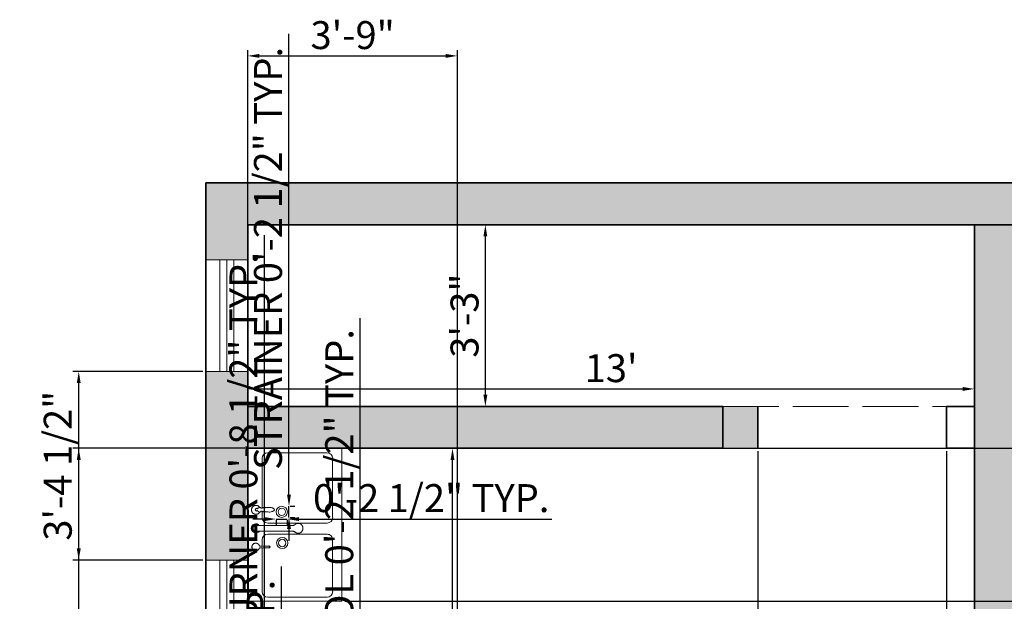
# Model space of a CAD drawing. Units: inches. Extents: x -40 to 424, y -33 to 568.
# Tile 6 of 8: x -40 to 171, y 438 to 563. Entities that reach past the tile are written whole.
import ezdxf

# ---------------------------------------------------------------- set-up
doc = ezdxf.new("R2010")
doc.units = ezdxf.units.IN
doc.linetypes.add('ACAD_ISO02W100', pattern=[15, 12, -3])
for name, color, linetype, lineweight in [('A-ANNO-DIMS', 7, 'Continuous', 18), ('A-FLOR-FIXT', 7, 'Continuous', 18), ('A-GLAZ', 7, 'Continuous', 18), ('A-WALL-OVHD', 7, 'ACAD_ISO02W100', 18), ('A-WALL-PATT', 30, 'Continuous', 13), ('wall', 7, 'Continuous', 35)]:
    doc.layers.add(name, color=color, linetype=linetype, lineweight=lineweight)
doc.styles.get("Standard").update_dxf_attribs({"font": 'arial.ttf'})
doc.dimstyles.new('ISO-25', dxfattribs={"dimtxt": 6, "dimasz": 2.5, "dimexe": 1.25, "dimexo": 0.625, "dimtad": 1, "dimdec": 1, "dimlunit": 3, "dimtxsty": 'Standard', "dimcen": 2.5, "dimadec": 0, "dimazin": 0, "dimtfac": 1, "dimtdec": 1, "dimtmove": 0, "dimatfit": 3, "dimfxl": 1, "dimarcsym": 0})

# ---------------------------------------------------------------- blocks, each defined once
blk = doc.blocks.new('*D27')
at = {"layer": 'A-ANNO-DIMS', "color": 0, "lineweight": -2, "transparency": 16777216}
for p, q in [((52.32, 471), (51.7, 471)), ((52.95, 281.5), (52.95, 468.5)), ((53.57, 279), (54.2, 279))]:
    blk.add_line(p, q, dxfattribs=at)
at = {"layer": 'A-ANNO-DIMS', "color": 0, "transparency": 16777216}
for points in [[(52.53, 468.5), (53.36, 468.5), (52.95, 471)], [(52.53, 281.5), (53.36, 281.5), (52.95, 279)]]:
    blk.add_solid(points, dxfattribs=at)
at = {"layer": 'Defpoints', "color": 0, "transparency": 16777216}
for p in [(52.95, 471), (52.95, 471), (52.95, 279)]:
    blk.add_point(p, dxfattribs=at)
at = {"layer": 'A-ANNO-DIMS', "color": 0, "transparency": 16777216, "insert": (49.26, 375), "char_height": 6, "attachment_point": 5, "rotation": 90}
blk.add_mtext("16'", dxfattribs=at)
blk = doc.blocks.new('*D28')
at = {"layer": 'A-ANNO-DIMS', "color": 0, "lineweight": -2, "transparency": 16777216}
for p, q in [((9.08, 457.74), (9.08, 411.34)), ((165, 457.74), (165, 411.34)), ((11.58, 412.59), (162.5, 412.59))]:
    blk.add_line(p, q, dxfattribs=at)
at = {"layer": 'A-ANNO-DIMS', "color": 0, "transparency": 16777216}
for points in [[(11.58, 413.01), (11.58, 412.18), (9.08, 412.59)], [(162.5, 413.01), (162.5, 412.18), (165, 412.59)]]:
    blk.add_solid(points, dxfattribs=at)
at = {"layer": 'Defpoints', "color": 0, "transparency": 16777216}
for p in [(9.08, 458.36), (165, 458.36), (165, 412.59)]:
    blk.add_point(p, dxfattribs=at)
at = {"layer": 'A-ANNO-DIMS', "color": 0, "transparency": 16777216, "insert": (87.04, 416.28), "char_height": 6, "attachment_point": 5}
blk.add_mtext('12\'-11.9"', dxfattribs=at)
blk = doc.blocks.new('*D29')
at = {"layer": 'A-ANNO-DIMS', "color": 0, "lineweight": -2, "transparency": 16777216}
for p, q in [((59.38, 519), (58.75, 519)), ((60, 482.5), (60, 516.5)), ((59.38, 480), (58.75, 480))]:
    blk.add_line(p, q, dxfattribs=at)
at = {"layer": 'A-ANNO-DIMS', "color": 0, "transparency": 16777216}
for points in [[(59.58, 516.5), (60.42, 516.5), (60, 519)], [(59.58, 482.5), (60.42, 482.5), (60, 480)]]:
    blk.add_solid(points, dxfattribs=at)
at = {"layer": 'Defpoints', "color": 0, "transparency": 16777216}
for p in [(60, 519), (60, 519), (60, 480)]:
    blk.add_point(p, dxfattribs=at)
at = {"layer": 'A-ANNO-DIMS', "color": 0, "transparency": 16777216, "insert": (56.31, 499.5), "char_height": 6, "attachment_point": 5, "rotation": 90}
blk.add_mtext('3\'-3"', dxfattribs=at)
blk = doc.blocks.new('*D30')
at = {"layer": 'A-ANNO-DIMS', "color": 0, "lineweight": -2, "transparency": 16777216}
for p, q in [((9, 510.87), (9, 482.5)), ((165, 510.87), (165, 482.5)), ((11.5, 483.75), (162.5, 483.75))]:
    blk.add_line(p, q, dxfattribs=at)
at = {"layer": 'A-ANNO-DIMS', "color": 0, "transparency": 16777216}
for points in [[(11.5, 484.17), (11.5, 483.33), (9, 483.75)], [(162.5, 484.17), (162.5, 483.33), (165, 483.75)]]:
    blk.add_solid(points, dxfattribs=at)
at = {"layer": 'Defpoints', "color": 0, "transparency": 16777216}
for p in [(9, 511.5), (165, 511.5), (165, 483.75)]:
    blk.add_point(p, dxfattribs=at)
at = {"layer": 'A-ANNO-DIMS', "color": 0, "transparency": 16777216, "insert": (87, 487.44), "char_height": 6, "attachment_point": 5}
blk.add_mtext("13'", dxfattribs=at)
blk = doc.blocks.new('WIN-48IN')
for p, q in [((0, 0), (0, 9)), ((48, 0), (48, 9)), ((0, 6), (48, 6)), ((0, 4.5), (48, 4.5)), ((0, 3), (48, 3))]:
    blk.add_line(p, q)
blk = doc.blocks.new('WIN-24IN')
for p, q in [((9, 24), (0, 24)), ((3, 0), (3, 24)), ((4.5, 0), (4.5, 24)), ((6, 0), (6, 24)), ((9, 0), (0, 0))]:
    blk.add_line(p, q)
blk = doc.blocks.new('SINK-STRAINER')
for radius in [1.2, 0.798]:
    blk.add_circle((1.2, 1.2), radius)
blk = doc.blocks.new('*D43')
at = {"layer": 'A-ANNO-DIMS', "color": 0, "lineweight": -2, "transparency": 16777216}
for p, q in [((16.2, 351), (16.2, 445.58)), ((9.62, 351), (17.45, 351)), ((16.2, 305.5), (16.2, 348.5)), ((9.62, 303), (17.45, 303))]:
    blk.add_line(p, q, dxfattribs=at)
at = {"layer": 'A-ANNO-DIMS', "color": 0, "transparency": 16777216}
for points in [[(15.78, 348.5), (16.62, 348.5), (16.2, 351)], [(15.78, 305.5), (16.62, 305.5), (16.2, 303)]]:
    blk.add_solid(points, dxfattribs=at)
at = {"layer": 'Defpoints', "color": 0, "transparency": 16777216}
for p in [(9, 351), (16.2, 351), (9, 303)]:
    blk.add_point(p, dxfattribs=at)
at = {"layer": 'A-ANNO-DIMS', "color": 0, "transparency": 16777216, "insert": (12.47, 399.54), "char_height": 6, "attachment_point": 5, "rotation": 90}
blk.add_mtext('WINDOW W1 4\'-0" TYP.', dxfattribs=at)
blk = doc.blocks.new('*D71')
at = {"layer": 'A-ANNO-DIMS', "color": 0, "lineweight": -2, "transparency": 16777216}
for p, q in [((33.12, 401.38), (33.12, 498.92)), ((32.88, 398.88), (31.88, 398.88)), ((33.12, 396.38), (33.12, 398.88)), ((32.88, 396.38), (31.88, 396.38)), ((33.12, 393.88), (33.12, 391.38))]:
    blk.add_line(p, q, dxfattribs=at)
at = {"layer": 'A-ANNO-DIMS', "color": 0, "transparency": 16777216}
for points in [[(32.71, 401.38), (33.54, 401.38), (33.12, 398.88)], [(32.71, 393.88), (33.54, 393.88), (33.12, 396.38)]]:
    blk.add_solid(points, dxfattribs=at)
at = {"layer": 'Defpoints', "color": 0, "transparency": 16777216}
for p in [(33.12, 398.88), (33.5, 398.88), (33.5, 396.38)]:
    blk.add_point(p, dxfattribs=at)
at = {"layer": 'A-ANNO-DIMS', "color": 0, "transparency": 16777216, "insert": (29.4, 451.4), "char_height": 6, "attachment_point": 5, "rotation": 90}
blk.add_mtext('CONTROL 0\'-2 1/2" TYP.', dxfattribs=at)
blk = doc.blocks.new('*D75')
at = {"layer": 'A-ANNO-DIMS', "color": 0, "lineweight": -2, "transparency": 16777216}
for p, q in [((12.57, 399.46), (12.57, 516.79)), ((13.25, 399.46), (11.32, 399.46)), ((12.57, 393.29), (12.57, 396.96)), ((13.25, 390.79), (11.32, 390.79))]:
    blk.add_line(p, q, dxfattribs=at)
at = {"layer": 'A-ANNO-DIMS', "color": 0, "transparency": 16777216}
for points in [[(12.15, 396.96), (12.99, 396.96), (12.57, 399.46)], [(12.15, 393.29), (12.99, 393.29), (12.57, 390.79)]]:
    blk.add_solid(points, dxfattribs=at)
at = {"layer": 'Defpoints', "color": 0, "transparency": 16777216}
for p in [(12.57, 399.46), (13.87, 399.46), (13.87, 390.79)]:
    blk.add_point(p, dxfattribs=at)
at = {"layer": 'A-ANNO-DIMS', "color": 0, "transparency": 16777216, "insert": (8.84, 459.38), "char_height": 6, "attachment_point": 5, "rotation": 90}
blk.add_mtext('REAR BURNER 0\'-8 1/2" TYP.', dxfattribs=at)
blk = doc.blocks.new('*D77')
at = {"layer": 'A-ANNO-DIMS', "color": 0, "lineweight": -2, "transparency": 16777216}
for p, q in [((17.84, 461.05), (17.84, 560.03)), ((17.84, 456.15), (17.84, 458.55)), ((18.11, 458.55), (19.09, 458.55)), ((18.11, 456.15), (19.09, 456.15)), ((17.84, 453.65), (17.84, 451.15))]:
    blk.add_line(p, q, dxfattribs=at)
at = {"layer": 'A-ANNO-DIMS', "color": 0, "transparency": 16777216}
for points in [[(17.42, 461.05), (18.26, 461.05), (17.84, 458.55)], [(17.42, 453.65), (18.26, 453.65), (17.84, 456.15)]]:
    blk.add_solid(points, dxfattribs=at)
at = {"layer": 'Defpoints', "color": 0, "transparency": 16777216}
for p in [(17.48, 458.55), (17.84, 458.55), (17.48, 456.15)]:
    blk.add_point(p, dxfattribs=at)
at = {"layer": 'A-ANNO-DIMS', "color": 0, "transparency": 16777216, "insert": (14.11, 511.79), "char_height": 6, "attachment_point": 5, "rotation": 90}
blk.add_mtext('STRAINER 0\'-2 1/2" TYP.', dxfattribs=at)
blk = doc.blocks.new('*D78')
at = {"layer": 'A-ANNO-DIMS', "color": 0, "lineweight": -2, "transparency": 16777216}
for p, q in [((12.59, 455.8), (10.09, 455.8)), ((15.09, 455.8), (17.48, 455.8)), ((15.09, 455.53), (15.09, 454.55)), ((17.48, 455.53), (17.48, 454.55)), ((19.98, 455.8), (74.29, 455.8))]:
    blk.add_line(p, q, dxfattribs=at)
at = {"layer": 'A-ANNO-DIMS', "color": 0, "transparency": 16777216}
for points in [[(12.59, 456.21), (12.59, 455.38), (15.09, 455.8)], [(19.98, 456.21), (19.98, 455.38), (17.48, 455.8)]]:
    blk.add_solid(points, dxfattribs=at)
at = {"layer": 'Defpoints', "color": 0, "transparency": 16777216}
for p in [(15.09, 456.15), (17.48, 456.15), (17.48, 455.8)]:
    blk.add_point(p, dxfattribs=at)
at = {"layer": 'A-ANNO-DIMS', "color": 0, "transparency": 16777216, "insert": (48.38, 459.52), "char_height": 6, "attachment_point": 5}
blk.add_mtext('0\'-2 1/2" TYP.', dxfattribs=at)
blk = doc.blocks.new('*D85')
at = {"layer": 'A-ANNO-DIMS', "color": 0, "lineweight": -2, "transparency": 16777216}
for p, q in [((-0.63, 487.5), (-28.55, 487.5)), ((-27.3, 449.5), (-27.3, 485)), ((-0.63, 447), (-28.55, 447))]:
    blk.add_line(p, q, dxfattribs=at)
at = {"layer": 'A-ANNO-DIMS', "color": 0, "transparency": 16777216}
for points in [[(-27.72, 485), (-26.88, 485), (-27.3, 487.5)], [(-27.72, 449.5), (-26.88, 449.5), (-27.3, 447)]]:
    blk.add_solid(points, dxfattribs=at)
at = {"layer": 'Defpoints', "color": 0, "transparency": 16777216}
for p in [(-27.3, 487.5), (0, 487.5), (0, 447)]:
    blk.add_point(p, dxfattribs=at)
at = {"layer": 'A-ANNO-DIMS', "color": 0, "transparency": 16777216, "insert": (-31.03, 467.25), "char_height": 6, "attachment_point": 5, "rotation": 90}
blk.add_mtext('3\'-4 1/2"', dxfattribs=at)
blk = doc.blocks.new('*D91')
at = {"layer": 'A-ANNO-DIMS', "color": 0, "lineweight": -2, "transparency": 16777216}
for p, q in [((9, 90.62), (9, 556.55)), ((54, 90.62), (54, 556.55)), ((11.5, 555.3), (51.5, 555.3))]:
    blk.add_line(p, q, dxfattribs=at)
at = {"layer": 'A-ANNO-DIMS', "color": 0, "transparency": 16777216}
for points in [[(11.5, 555.72), (11.5, 554.88), (9, 555.3)], [(51.5, 555.72), (51.5, 554.88), (54, 555.3)]]:
    blk.add_solid(points, dxfattribs=at)
at = {"layer": 'Defpoints', "color": 0, "transparency": 16777216}
for p in [(54, 555.3), (9, 90), (54, 90)]:
    blk.add_point(p, dxfattribs=at)
at = {"layer": 'A-ANNO-DIMS', "color": 0, "transparency": 16777216, "insert": (31.5, 558.99), "char_height": 6, "attachment_point": 5}
blk.add_mtext('3\'-9"', dxfattribs=at)
blk = doc.blocks.new('*D92')
at = {"layer": 'A-ANNO-DIMS', "color": 0, "lineweight": -2, "transparency": 16777216}
for p, q in [((118.47, 470.38), (118.47, -28.55)), ((159, 470.38), (159, -28.55)), ((120.97, -27.3), (156.5, -27.3))]:
    blk.add_line(p, q, dxfattribs=at)
at = {"layer": 'A-ANNO-DIMS', "color": 0, "transparency": 16777216}
for points in [[(120.97, -26.88), (120.97, -27.72), (118.47, -27.3)], [(156.5, -26.88), (156.5, -27.72), (159, -27.3)]]:
    blk.add_solid(points, dxfattribs=at)
at = {"layer": 'Defpoints', "color": 0, "transparency": 16777216}
for p in [(118.47, 471), (159, 471), (159, -27.3)]:
    blk.add_point(p, dxfattribs=at)
at = {"layer": 'A-ANNO-DIMS', "color": 0, "transparency": 16777216, "insert": (138.73, -23.57), "char_height": 6, "attachment_point": 5}
blk.add_mtext('3\'-4 1/2"', dxfattribs=at)
blk = doc.blocks.new('*D100')
at = {"layer": 'A-ANNO-DIMS', "color": 0, "lineweight": -2, "transparency": 16777216}
for p, q in [((8.37, 471), (-28.55, 471)), ((-27.3, 360.94), (-27.3, 468.5)), ((8.37, 358.44), (-28.55, 358.44))]:
    blk.add_line(p, q, dxfattribs=at)
at = {"layer": 'A-ANNO-DIMS', "color": 0, "transparency": 16777216}
for points in [[(-27.72, 468.5), (-26.88, 468.5), (-27.3, 471)], [(-27.72, 360.94), (-26.88, 360.94), (-27.3, 358.44)]]:
    blk.add_solid(points, dxfattribs=at)
at = {"layer": 'Defpoints', "color": 0, "transparency": 16777216}
for p in [(-27.3, 471), (9, 471), (9, 358.44)]:
    blk.add_point(p, dxfattribs=at)
at = {"layer": 'A-ANNO-DIMS', "color": 0, "transparency": 16777216, "insert": (-31.03, 414.72), "char_height": 6, "attachment_point": 5, "rotation": 90}
blk.add_mtext('9\'-4 1/2"', dxfattribs=at)
blk = doc.blocks.new('*D102')
at = {"layer": 'A-ANNO-DIMS', "color": 0, "lineweight": -2, "transparency": 16777216}
for p, q in [((29.83, 471), (412.55, 471)), ((411.3, 440.63), (411.3, 468.5)), ((29.83, 438.13), (412.55, 438.13))]:
    blk.add_line(p, q, dxfattribs=at)
at = {"layer": 'A-ANNO-DIMS', "color": 0, "transparency": 16777216}
for points in [[(410.88, 468.5), (411.72, 468.5), (411.3, 471)], [(410.88, 440.63), (411.72, 440.63), (411.3, 438.13)]]:
    blk.add_solid(points, dxfattribs=at)
at = {"layer": 'Defpoints', "color": 0, "transparency": 16777216}
for p in [(29.21, 471), (411.3, 471), (29.21, 438.13)]:
    blk.add_point(p, dxfattribs=at)
at = {"layer": 'A-ANNO-DIMS', "color": 0, "transparency": 16777216, "insert": (407.61, 454.56), "char_height": 6, "attachment_point": 5, "rotation": 90}
blk.add_mtext('2\'-9"', dxfattribs=at)

msp = doc.modelspace()

# ---------------------------------------------------------------- hatches: boundary and pattern name
at = {"layer": 'A-WALL-PATT'}
h = msp.add_hatch(color=256, dxfattribs=at)
h.dxf.hatch_style = 1
h.paths.add_polyline_path([(9, 399), (0, 399), (0, 351), (9, 351)])
h.paths.add_polyline_path([(9, 303), (0, 303), (0, 210), (9, 210)])
h.paths.add_polyline_path([(9, 150), (0, 150), (0, 0), (384, 0), (384, 69), (375, 69), (375, 62.24), (375, 9), (9, 9)])
h.paths.add_polyline_path([(210, 177), (216, 177), (216, 186), (210, 186), (210, 216), (201, 216), (201, 90), (195, 90), (195, 81), (201, 81), (201, 9), (210, 9)])
h.paths.add_polyline_path([(384, 216), (375, 216), (375, 117), (384, 117)])
h.paths.add_polyline_path([(384, 298.5), (375, 298.5), (375, 279), (375, 240), (384, 240)])
h.paths.add_polyline_path([(384, 417), (375, 417), (375, 334.5), (384, 334.5)])
h.paths.add_polyline_path([(384, 528), (216, 528), (216, 519), (375, 519), (375, 465), (384, 465)])
h.paths.add_polyline_path([(192, 528), (0, 528), (0, 511.5), (9, 511.5), (9, 519), (192, 519)])
h.paths.add_polyline_path([(9, 487.5), (0, 487.5), (0, 447), (9, 447)])
h.paths.add_polyline_path([(111, 480), (9, 480), (9, 471), (111, 471)])
h.paths.add_polyline_path([(174, 519), (165, 519), (165, 354), (174, 354)])
h.paths.add_polyline_path([(243, 426), (237.86, 426), (234, 426), (234, 420), (174, 420), (174, 411), (234, 411), (234, 405), (239.14, 405), (243, 405)])
h.paths.add_polyline_path([(243, 519), (234, 519), (234, 460.14, -0.031638), (237.86, 460.2), (237.86, 462), (243, 462)])
h.paths.add_polyline_path([(243, 369), (234, 369), (234, 354), (375, 354), (375, 363), (243, 363)])
h.paths.add_polyline_path([(375, 279), (195, 279), (195, 270), (201, 270), (201, 264), (210, 264), (210, 270), (375, 270)])
h.paths.add_polyline_path([(291, 270), (282, 270), (282, 222), (286.29, 222), (291, 222)])
h.paths.add_polyline_path([(375, 186), (291, 186), (291, 192), (282, 192), (282, 186), (252, 186), (252, 180.86), (252, 177), (375, 177)])
h.paths.add_polyline_path([(147, 279), (9, 279), (9, 270), (147, 270)])
h = msp.add_hatch(color=256, dxfattribs=at)
h.dxf.hatch_style = 1
h.paths.add_polyline_path([(118.47, 480), (111, 480), (111, 471), (118.47, 471)])

# ---------------------------------------------------------------- linework, layer by layer
at = {"layer": 'A-FLOR-FIXT'}
for p, q in [((13.29, 470.05), (22.39, 470.05)), ((22.39, 470.05), (26.02, 470.05)), ((12.09, 458.15), (12.09, 468.85)), ((27.21, 468.85), (27.21, 456.13)), ((10.64, 457.91), (10.58, 457.81)), ((10.58, 457.81), (10.58, 457.81)), ((10.64, 457.71), (10.58, 457.81)), ((10.58, 457.81), (10.58, 457.81)), ((10.58, 457.81), (10.58, 457.81)), ((10.66, 457.93), (10.64, 457.91)), ((10.66, 457.69), (10.64, 457.71)), ((10.82, 458.05), (10.66, 457.93)), ((10.82, 457.57), (10.66, 457.69)), ((10.83, 458.05), (10.82, 458.05)), ((10.83, 457.56), (10.82, 457.57)), ((10.88, 458.09), (10.83, 458.05)), ((10.88, 457.53), (10.83, 457.56)), ((10.93, 458.11), (10.88, 458.09)), ((10.93, 457.51), (10.88, 457.53)), ((11, 458.05), (10.93, 458.11)), ((11, 457.56), (10.93, 457.51)), ((11.01, 458.05), (11, 458.05)), ((11.01, 457.57), (11, 457.56)), ((11.06, 458.01), (11.01, 458.05)), ((11.06, 457.61), (11.01, 457.57)), ((11.07, 458.01), (11.06, 458.01)), ((11.07, 457.61), (11.06, 457.61)), ((11.11, 458.01), (11.07, 458.01)), ((11.11, 457.61), (11.07, 457.61)), ((11.17, 458.1), (11.11, 458.01)), ((11.17, 457.52), (11.11, 457.61)), ((11.21, 458.16), (11.17, 458.1)), ((11.21, 457.46), (11.17, 457.52)), ((11.24, 458.2), (11.21, 458.16)), ((11.24, 457.42), (11.21, 457.46)), ((11.26, 458.22), (11.24, 458.21)), ((11.24, 458.21), (11.24, 458.2)), ((11.24, 457.41), (11.24, 457.42)), ((11.26, 457.4), (11.24, 457.41)), ((11.27, 458.22), (11.26, 458.22)), ((11.27, 457.4), (11.26, 457.4)), ((11.41, 458.28), (11.27, 458.22)), ((11.41, 457.34), (11.27, 457.4)), ((11.46, 458.31), (11.41, 458.28)), ((11.42, 457.33), (11.41, 457.34)), ((11.43, 457.33), (11.42, 457.33)), ((11.42, 457.33), (11.42, 457.33)), ((11.46, 457.31), (11.43, 457.33)), ((11.46, 458.31), (11.46, 458.31)), ((11.65, 458.28), (11.46, 458.31)), ((11.65, 457.34), (11.46, 457.31)), ((11.46, 457.31), (11.46, 457.31)), ((11.46, 457.31), (11.46, 457.31)), ((11.66, 458.28), (11.65, 458.28)), ((11.66, 457.34), (11.65, 457.34)), ((11.68, 458.28), (11.66, 458.28)), ((11.68, 457.34), (11.66, 457.34)), ((11.7, 458.28), (11.68, 458.28)), ((11.7, 457.34), (11.68, 457.34)), ((11.86, 458.15), (11.7, 458.28)), ((11.89, 457.49), (11.7, 457.34)), ((11.89, 458.13), (11.86, 458.15)), ((11.99, 458.12), (11.89, 458.13)), ((11.95, 457.49), (11.89, 457.49)), ((11.99, 457.49), (11.95, 457.49)), ((12.1, 458.16), (11.99, 458.12)), ((12.08, 457.47), (11.99, 457.49)), ((12.1, 457.46), (12.08, 457.47)), ((12.09, 456.13), (12.09, 457.46)), ((12.18, 458.18), (12.1, 458.16)), ((12.18, 457.44), (12.1, 457.46)), ((12.26, 458.27), (12.18, 458.18)), ((12.26, 457.35), (12.18, 457.44)), ((12.29, 458.27), (12.26, 458.27)), ((12.29, 457.35), (12.26, 457.35)), ((12.4, 458.19), (12.29, 458.27)), ((12.4, 457.43), (12.29, 457.35)), ((12.29, 457.35), (12.29, 457.35)), ((12.46, 458.2), (12.4, 458.19)), ((12.63, 457.39), (12.4, 457.43)), ((12.58, 458.22), (12.46, 458.2)), ((12.6, 458.22), (12.58, 458.22)), ((12.64, 458.23), (12.6, 458.22)), ((12.71, 457.38), (12.63, 457.39)), ((12.66, 458.23), (12.64, 458.23)), ((12.71, 458.24), (12.66, 458.23)), ((12.72, 458.24), (12.71, 458.24)), ((12.75, 457.37), (12.71, 457.38)), ((12.76, 458.25), (12.72, 458.24)), ((12.79, 457.36), (12.75, 457.37)), ((12.81, 458.26), (12.76, 458.25)), ((12.87, 457.35), (12.79, 457.36)), ((12.9, 458.27), (12.81, 458.26)), ((12.88, 457.35), (12.87, 457.35)), ((12.9, 457.35), (12.88, 457.35)), ((12.94, 458.28), (12.9, 458.27)), ((12.93, 457.34), (12.9, 457.35)), ((12.94, 457.34), (12.93, 457.34)), ((13.36, 458.3), (12.94, 458.28)), ((13.04, 457.34), (12.94, 457.34)), ((13.05, 457.34), (13.04, 457.34)), ((13.08, 457.33), (13.05, 457.34)), ((13.26, 457.32), (13.08, 457.33)), ((13.36, 457.32), (13.26, 457.32)), ((13.37, 458.3), (13.36, 458.3)), ((13.58, 457.31), (13.36, 457.32)), ((13.51, 458.3), (13.37, 458.3)), ((13.52, 458.3), (13.51, 458.3)), ((13.55, 458.31), (13.52, 458.3)), ((13.7, 458.31), (13.55, 458.31)), ((13.7, 457.31), (13.58, 457.31)), ((13.7, 458.31), (13.7, 458.31)), ((13.78, 458.3), (13.7, 458.31)), ((14.02, 457.36), (13.7, 457.31)), ((13.79, 458.29), (13.78, 458.3)), ((13.83, 458.29), (13.79, 458.29)), ((13.79, 458.29), (13.79, 458.29)), ((13.85, 458.28), (13.83, 458.29)), ((14.02, 458.26), (13.85, 458.28)), ((14.13, 458.23), (14.02, 458.26)), ((14.16, 457.4), (14.02, 457.36)), ((14.22, 458.2), (14.13, 458.23)), ((14.27, 457.43), (14.16, 457.4)), ((14.27, 458.19), (14.22, 458.2)), ((14.37, 458.14), (14.27, 458.19)), ((14.51, 457.53), (14.27, 457.43)), ((14.46, 458.11), (14.37, 458.14)), ((14.51, 458.09), (14.46, 458.11)), ((14.6, 458.01), (14.51, 458.09)), ((14.58, 457.59), (14.51, 457.53)), ((14.68, 457.67), (14.58, 457.59)), ((14.65, 457.98), (14.6, 458.01)), ((14.68, 457.95), (14.65, 457.98)), ((14.69, 457.89), (14.68, 457.95)), ((14.69, 457.7), (14.68, 457.67)), ((14.71, 457.81), (14.69, 457.89)), ((14.7, 457.77), (14.69, 457.7)), ((14.71, 457.81), (14.7, 457.77)), ((22.39, 454.93), (13.29, 454.93)), ((26.02, 454.93), (22.39, 454.93)), ((10.7, 454.4), (10.83, 454.4)), ((10.73, 453.22), (10.81, 453.22)), ((10.81, 453.22), (10.83, 453.22)), ((10.83, 454.4), (10.86, 454.4)), ((10.83, 453.22), (10.86, 453.22)), ((10.86, 454.4), (10.94, 454.4)), ((10.86, 453.22), (10.94, 453.22)), ((10.94, 454.4), (11, 454.4)), ((10.94, 453.22), (10.95, 453.22)), ((10.95, 453.22), (10.96, 453.22)), ((10.96, 453.22), (11, 453.22)), ((11, 454.4), (11.02, 454.4)), ((11, 453.22), (11.02, 453.22)), ((11.02, 454.4), (11.15, 454.4)), ((11.02, 453.22), (11.15, 453.22)), ((11.15, 454.4), (11.29, 454.4)), ((11.15, 453.22), (11.29, 453.22)), ((11.29, 454.4), (11.31, 454.4)), ((11.29, 453.22), (11.3, 453.22)), ((11.3, 453.22), (11.31, 453.22)), ((11.32, 454.41), (11.31, 454.4)), ((11.31, 454.4), (11.31, 454.4)), ((11.31, 453.22), (11.32, 453.22)), ((11.32, 454.41), (11.36, 454.4)), ((11.32, 453.22), (11.36, 453.22)), ((11.35, 454.41), (11.36, 454.4)), ((11.36, 454.4), (11.36, 454.4)), ((11.36, 454.4), (11.38, 454.4)), ((11.36, 453.22), (11.38, 453.22)), ((11.38, 454.4), (11.42, 454.4)), ((11.38, 453.22), (11.42, 453.22)), ((11.42, 454.4), (11.46, 454.4)), ((11.42, 453.22), (11.46, 453.22)), ((11.46, 454.4), (11.48, 454.4)), ((11.46, 453.22), (11.48, 453.22)), ((11.48, 454.4), (11.49, 454.4)), ((11.48, 453.22), (11.49, 453.22)), ((11.49, 454.42), (11.49, 454.4)), ((11.49, 454.4), (12.15, 454.4)), ((11.49, 454.4), (11.49, 454.4)), ((11.49, 454.4), (11.49, 454.4)), ((11.49, 453.22), (11.49, 453.22)), ((11.49, 453.22), (11.49, 453.22)), ((11.49, 453.22), (11.71, 453.22)), ((11.71, 453.22), (14.77, 453.22)), ((12.15, 454.4), (12.39, 454.4)), ((12.39, 454.4), (13.02, 454.4)), ((13.02, 454.4), (13.03, 454.4)), ((13.03, 454.4), (13.11, 454.4)), ((13.11, 454.4), (13.13, 454.4)), ((13.13, 454.4), (13.14, 454.4)), ((13.14, 454.4), (13.16, 454.4)), ((13.16, 454.4), (13.16, 454.4)), ((13.16, 454.4), (13.17, 454.4)), ((13.17, 454.4), (13.25, 454.4)), ((13.25, 454.4), (13.26, 454.4)), ((13.26, 454.4), (13.3, 454.4)), ((22.39, 452.54), (13.29, 452.54)), ((13.3, 454.4), (13.31, 454.4)), ((13.31, 454.4), (13.33, 454.4)), ((13.33, 454.4), (13.47, 454.4)), ((13.47, 454.4), (13.48, 454.4)), ((13.48, 454.4), (13.61, 454.4)), ((13.61, 454.4), (13.61, 454.4)), ((13.61, 454.4), (13.69, 454.4)), ((13.69, 454.4), (13.78, 454.4)), ((13.78, 454.4), (14.05, 454.4)), ((14.05, 454.4), (14.06, 454.4)), ((14.06, 454.4), (14.1, 454.4)), ((14.1, 454.4), (14.12, 454.4)), ((14.12, 454.4), (14.13, 454.4)), ((14.13, 454.4), (14.2, 454.4)), ((14.2, 454.4), (14.26, 454.4)), ((14.26, 454.4), (14.28, 454.4)), ((14.28, 454.4), (14.32, 454.4)), ((14.32, 454.4), (14.46, 454.4)), ((14.46, 454.4), (14.6, 454.4)), ((14.6, 454.4), (14.76, 454.4)), ((14.76, 454.4), (14.91, 454.4)), ((14.77, 453.22), (14.84, 453.22)), ((14.84, 453.22), (15.04, 453.22)), ((14.91, 454.4), (15.06, 454.4)), ((15.04, 453.22), (15.11, 453.22)), ((15.06, 454.4), (15.32, 454.4)), ((15.11, 453.22), (15.19, 453.22)), ((15.19, 453.22), (15.26, 453.22)), ((15.26, 453.22), (15.5, 453.22)), ((15.32, 454.4), (15.52, 454.4)), ((15.5, 453.22), (15.52, 453.22)), ((15.52, 454.4), (15.55, 454.4)), ((15.52, 453.22), (15.69, 453.22)), ((15.55, 454.4), (15.77, 454.4)), ((15.69, 453.22), (16.35, 453.22)), ((15.77, 454.4), (16.06, 454.4)), ((16.06, 454.4), (16.11, 454.4)), ((16.11, 454.4), (16.69, 454.4)), ((16.35, 453.22), (16.69, 453.22)), ((16.69, 454.4), (17.68, 454.4)), ((16.69, 453.22), (16.86, 453.22)), ((16.86, 453.22), (17.2, 453.22)), ((17.2, 453.22), (17.71, 453.22)), ((17.68, 454.4), (17.69, 454.4)), ((17.69, 454.4), (17.71, 454.4)), ((17.71, 454.4), (18.52, 454.4)), ((17.71, 453.22), (18.32, 453.22)), ((22.39, 452.54), (26.02, 452.54)), ((26.02, 452.54), (22.39, 452.54)), ((12.09, 451.34), (12.09, 449.98)), ((27.21, 440.21), (27.21, 451.34)), ((27.21, 451.34), (27.21, 449.69)), ((11.7, 449.98), (11.64, 449.98)), ((11.7, 449.64), (11.64, 449.64)), ((11.71, 449.98), (11.7, 449.98)), ((11.71, 449.64), (11.7, 449.64)), ((11.77, 449.98), (11.71, 449.98)), ((11.77, 449.64), (11.71, 449.64)), ((11.82, 449.98), (11.77, 449.98)), ((11.99, 449.64), (11.77, 449.64)), ((11.9, 449.98), (11.82, 449.98)), ((12.03, 449.98), (11.9, 449.98)), ((12.03, 449.64), (11.99, 449.64)), ((12.31, 449.98), (12.03, 449.98)), ((12.05, 449.64), (12.03, 449.64)), ((12.35, 449.64), (12.05, 449.64)), ((12.09, 449.64), (12.09, 440.21)), ((12.35, 449.98), (12.31, 449.98)), ((12.64, 449.98), (12.35, 449.98)), ((12.62, 449.64), (12.35, 449.64)), ((12.64, 449.64), (12.62, 449.64)), ((12.69, 449.98), (12.64, 449.98)), ((12.67, 449.64), (12.64, 449.64)), ((12.72, 449.64), (12.67, 449.64)), ((12.72, 449.98), (12.69, 449.98)), ((12.78, 449.98), (12.72, 449.98)), ((12.82, 449.64), (12.72, 449.64)), ((12.85, 449.98), (12.78, 449.98)), ((12.9, 449.64), (12.82, 449.64)), ((12.82, 449.64), (12.82, 449.64)), ((12.82, 449.64), (12.82, 449.64)), ((12.87, 449.98), (12.85, 449.98)), ((12.96, 449.98), (12.87, 449.98)), ((12.95, 449.64), (12.9, 449.64)), ((12.97, 449.64), (12.95, 449.64)), ((12.97, 449.98), (12.96, 449.98)), ((12.98, 449.98), (12.97, 449.98)), ((13.04, 449.64), (12.97, 449.64)), ((13.1, 449.98), (12.98, 449.98)), ((13.18, 449.64), (13.04, 449.64)), ((13.27, 449.98), (13.1, 449.98)), ((13.2, 449.64), (13.18, 449.64)), ((13.24, 449.64), (13.2, 449.64)), ((13.27, 449.64), (13.24, 449.64)), ((13.27, 449.98), (13.27, 449.98)), ((13.33, 449.98), (13.27, 449.98)), ((13.28, 449.64), (13.27, 449.64)), ((13.47, 449.64), (13.28, 449.64)), ((13.35, 449.98), (13.33, 449.98)), ((13.37, 449.98), (13.35, 449.98)), ((13.47, 449.98), (13.37, 449.98)), ((13.47, 449.98), (13.48, 450)), ((13.48, 449.98), (13.47, 449.98)), ((13.48, 449.62), (13.47, 449.64)), ((13.47, 449.64), (13.47, 449.64)), ((13.48, 449.64), (13.47, 449.64)), ((13.48, 450), (13.57, 450.03)), ((13.51, 449.98), (13.48, 449.98)), ((13.51, 449.64), (13.48, 449.64)), ((13.57, 449.6), (13.48, 449.62)), ((13.53, 449.98), (13.51, 449.98)), ((13.53, 449.64), (13.51, 449.64)), ((13.29, 439.01), (22.39, 439.01)), ((22.39, 439.01), (26.02, 439.01))]:
    msp.add_line(p, q, dxfattribs=at)
msp.add_lwpolyline([(9, 438.13), (9, 471), (22.39, 471), (29.21, 471), (29.21, 438.13), (22.39, 438.13)], close=True, dxfattribs=at)
for points in [[(11.56, 458.29), (11.53, 458.33), (11.5, 458.37), (11.46, 458.42), (11.42, 458.46), (11.37, 458.5), (11.32, 458.54), (11.27, 458.57), (11.22, 458.61), (11.16, 458.64), (11.11, 458.66), (11.05, 458.68), (10.99, 458.7), (10.93, 458.72), (10.87, 458.73), (10.8, 458.73), (10.74, 458.73), (10.68, 458.73), (10.61, 458.73), (10.55, 458.72), (10.49, 458.7), (10.43, 458.68), (10.37, 458.66), (10.32, 458.64), (10.26, 458.61), (10.21, 458.57), (10.16, 458.54), (10.11, 458.5), (10.06, 458.45), (10.02, 458.41), (9.98, 458.36), (9.94, 458.31), (9.91, 458.25), (9.88, 458.2), (9.85, 458.14), (9.83, 458.08), (9.81, 458.02), (9.8, 457.96), (9.79, 457.9), (9.78, 457.84), (9.78, 457.77), (9.78, 457.71), (9.79, 457.65), (9.8, 457.59), (9.81, 457.53), (9.83, 457.47), (9.85, 457.41), (9.88, 457.35), (9.91, 457.29), (9.94, 457.24), (9.98, 457.19), (10.02, 457.14), (10.06, 457.1), (10.11, 457.05), (10.16, 457.01), (10.21, 456.98), (10.26, 456.94), (10.32, 456.91), (10.37, 456.89), (10.43, 456.87), (10.49, 456.85), (10.55, 456.83), (10.61, 456.82), (10.68, 456.82), (10.74, 456.81), (10.8, 456.82), (10.87, 456.82), (10.93, 456.83), (10.99, 456.85), (11.05, 456.87), (11.11, 456.89), (11.16, 456.91), (11.22, 456.94), (11.27, 456.98), (11.32, 457.01), (11.37, 457.05), (11.42, 457.09), (11.46, 457.13), (11.5, 457.18), (11.53, 457.22), (11.56, 457.26), (11.59, 457.3), (11.6, 457.33)], [(11.35, 454.41), (11.34, 454.42), (11.32, 454.44), (11.28, 454.47), (11.24, 454.49), (11.2, 454.52), (11.15, 454.55), (11.1, 454.58), (11.06, 454.6), (11.01, 454.62), (10.96, 454.64), (10.92, 454.65), (10.87, 454.66), (10.83, 454.67), (10.78, 454.68), (10.74, 454.68), (10.7, 454.68), (10.66, 454.68), (10.61, 454.68), (10.57, 454.67), (10.53, 454.67), (10.49, 454.66), (10.45, 454.64), (10.4, 454.63), (10.36, 454.62), (10.33, 454.6), (10.29, 454.58), (10.25, 454.56), (10.21, 454.54), (10.18, 454.51), (10.15, 454.48), (10.11, 454.46), (10.08, 454.43), (10.05, 454.4), (10.02, 454.36), (10, 454.33), (9.97, 454.29), (9.95, 454.26), (9.93, 454.22), (9.91, 454.18), (9.89, 454.14), (9.88, 454.1), (9.86, 454.06), (9.85, 454.02), (9.84, 453.98), (9.84, 453.94), (9.83, 453.9), (9.83, 453.85), (9.83, 453.81), (9.83, 453.77), (9.83, 453.73), (9.84, 453.68), (9.84, 453.64), (9.85, 453.6), (9.86, 453.56), (9.88, 453.52), (9.89, 453.48), (9.91, 453.44), (9.93, 453.4), (9.95, 453.36), (9.97, 453.33), (10, 453.29), (10.02, 453.26), (10.05, 453.23), (10.08, 453.19), (10.11, 453.17), (10.15, 453.14), (10.18, 453.11), (10.21, 453.09), (10.25, 453.06), (10.29, 453.04), (10.33, 453.02), (10.36, 453.01), (10.4, 452.99), (10.45, 452.98), (10.49, 452.97), (10.53, 452.96), (10.57, 452.95), (10.61, 452.94), (10.66, 452.94), (10.7, 452.94), (10.74, 452.94), (10.78, 452.94), (10.83, 452.95), (10.87, 452.96), (10.92, 452.97), (10.96, 452.98), (11.01, 453), (11.06, 453.02), (11.1, 453.05), (11.15, 453.07), (11.2, 453.1), (11.24, 453.13), (11.28, 453.15), (11.32, 453.18), (11.34, 453.2), (11.36, 453.22)], [(18.52, 454.4), (18.64, 454.41), (18.74, 454.42), (18.83, 454.43), (18.89, 454.45), (18.94, 454.48), (18.98, 454.5), (19.01, 454.52), (19.03, 454.54), (19.05, 454.56), (19.06, 454.57), (19.07, 454.58), (19.08, 454.59), (19.09, 454.59), (19.1, 454.6), (19.11, 454.61), (19.12, 454.62), (19.14, 454.63), (19.15, 454.64), (19.17, 454.66), (19.19, 454.67), (19.21, 454.69), (19.24, 454.71), (19.25, 454.72), (19.27, 454.73), (19.28, 454.74), (19.3, 454.75), (19.31, 454.76), (19.31, 454.76), (19.32, 454.77), (19.33, 454.77), (19.35, 454.78), (19.36, 454.78), (19.38, 454.79), (19.4, 454.8), (19.42, 454.81), (19.45, 454.82), (19.48, 454.82), (19.51, 454.83), (19.55, 454.84), (19.59, 454.85), (19.63, 454.86), (19.67, 454.87), (19.72, 454.87), (19.78, 454.88), (19.85, 454.88), (19.92, 454.87), (20, 454.86), (20.1, 454.85)], [(20.81, 453.51), (20.81, 453.51), (20.81, 453.51), (20.81, 453.52), (20.81, 453.52), (20.81, 453.53), (20.81, 453.53), (20.82, 453.55), (20.82, 453.56), (20.82, 453.58), (20.82, 453.6), (20.83, 453.63), (20.83, 453.66), (20.83, 453.69), (20.84, 453.72), (20.84, 453.76), (20.84, 453.79), (20.84, 453.83), (20.84, 453.86), (20.84, 453.89), (20.84, 453.92), (20.83, 453.95), (20.83, 453.98), (20.83, 454), (20.83, 454.02), (20.83, 454.04), (20.82, 454.05), (20.82, 454.06), (20.82, 454.06), (20.82, 454.07), (20.82, 454.07), (20.82, 454.07), (20.82, 454.07), (20.82, 454.07), (20.82, 454.07), (20.82, 454.07), (20.82, 454.08), (20.82, 454.08), (20.82, 454.09), (20.81, 454.1), (20.81, 454.12), (20.8, 454.13), (20.79, 454.16), (20.78, 454.18), (20.77, 454.21), (20.76, 454.23), (20.75, 454.26), (20.73, 454.29), (20.72, 454.32), (20.7, 454.35), (20.69, 454.38), (20.67, 454.4), (20.66, 454.42), (20.64, 454.44), (20.63, 454.46), (20.62, 454.48), (20.61, 454.49), (20.6, 454.51), (20.59, 454.52), (20.59, 454.52), (20.58, 454.53), (20.58, 454.53), (20.58, 454.54), (20.58, 454.54), (20.57, 454.54), (20.57, 454.55), (20.57, 454.55), (20.57, 454.55), (20.56, 454.56), (20.56, 454.56), (20.55, 454.57), (20.54, 454.58), (20.53, 454.59), (20.51, 454.6), (20.49, 454.62), (20.47, 454.63), (20.45, 454.65), (20.43, 454.67), (20.41, 454.68), (20.39, 454.7), (20.37, 454.72), (20.35, 454.73), (20.33, 454.74), (20.31, 454.75), (20.28, 454.77), (20.25, 454.78), (20.21, 454.8), (20.16, 454.82), (20.1, 454.85)], [(11.02, 454.4), (11, 454.42), (10.96, 454.43), (10.93, 454.44), (10.89, 454.45), (10.85, 454.46), (10.8, 454.47), (10.76, 454.47), (10.72, 454.47), (10.68, 454.48), (10.64, 454.47), (10.61, 454.47), (10.57, 454.47), (10.54, 454.46), (10.5, 454.45), (10.47, 454.44), (10.44, 454.43), (10.41, 454.41), (10.38, 454.4), (10.35, 454.38), (10.33, 454.37), (10.3, 454.35), (10.27, 454.33), (10.25, 454.31), (10.23, 454.28), (10.2, 454.26), (10.18, 454.23), (10.16, 454.21), (10.14, 454.18), (10.13, 454.15), (10.11, 454.13), (10.09, 454.1), (10.08, 454.07), (10.07, 454.04), (10.06, 454), (10.05, 453.97), (10.04, 453.94), (10.04, 453.91), (10.03, 453.88), (10.03, 453.84), (10.03, 453.81), (10.03, 453.78), (10.03, 453.75), (10.04, 453.71), (10.04, 453.68), (10.05, 453.65), (10.06, 453.62), (10.07, 453.59), (10.08, 453.56), (10.09, 453.53), (10.11, 453.5), (10.13, 453.47), (10.14, 453.44), (10.16, 453.41), (10.18, 453.39), (10.2, 453.36), (10.23, 453.34), (10.25, 453.32), (10.27, 453.29), (10.3, 453.27), (10.33, 453.26), (10.35, 453.24), (10.38, 453.22), (10.41, 453.21), (10.44, 453.19), (10.47, 453.18), (10.5, 453.17), (10.54, 453.16), (10.57, 453.16), (10.61, 453.15), (10.64, 453.15), (10.68, 453.15), (10.72, 453.15), (10.76, 453.15), (10.8, 453.15), (10.85, 453.16), (10.89, 453.17), (10.93, 453.18), (10.96, 453.19), (11, 453.2), (11.02, 453.22)], [(10.7, 454.4), (10.62, 454.39), (10.55, 454.37), (10.49, 454.35), (10.44, 454.32), (10.4, 454.3), (10.36, 454.28), (10.33, 454.25), (10.31, 454.23), (10.28, 454.21), (10.26, 454.18), (10.24, 454.16), (10.22, 454.13), (10.2, 454.11), (10.19, 454.08), (10.18, 454.06), (10.16, 454.03), (10.15, 454.01), (10.15, 453.98), (10.14, 453.95), (10.13, 453.92), (10.13, 453.9), (10.12, 453.87), (10.12, 453.84), (10.12, 453.81), (10.12, 453.78), (10.12, 453.75), (10.13, 453.73), (10.13, 453.7), (10.14, 453.67), (10.15, 453.64), (10.16, 453.61), (10.18, 453.57), (10.19, 453.54), (10.21, 453.51), (10.24, 453.47), (10.27, 453.43), (10.3, 453.4), (10.35, 453.35), (10.41, 453.31), (10.47, 453.26)], [(10.47, 453.26), (10.7, 453.22), (10.71, 453.22), (10.71, 453.22), (10.72, 453.22), (10.73, 453.22)], [(20.81, 453.51), (20.77, 453.42), (20.73, 453.34), (20.7, 453.28), (20.66, 453.22), (20.63, 453.17), (20.6, 453.13), (20.58, 453.1), (20.55, 453.07), (20.53, 453.04), (20.5, 453.02), (20.48, 453), (20.46, 452.98), (20.44, 452.97), (20.43, 452.95), (20.41, 452.94), (20.4, 452.93), (20.38, 452.92), (20.37, 452.91), (20.36, 452.9), (20.35, 452.9), (20.34, 452.89), (20.33, 452.88), (20.32, 452.87), (20.31, 452.87), (20.29, 452.86), (20.28, 452.86), (20.27, 452.85), (20.26, 452.84), (20.24, 452.84), (20.23, 452.83), (20.21, 452.83), (20.2, 452.82), (20.18, 452.81), (20.16, 452.81), (20.15, 452.8), (20.13, 452.79), (20.11, 452.79), (20.08, 452.78), (20.06, 452.77), (20.04, 452.77), (20.01, 452.76), (19.98, 452.76), (19.95, 452.75), (19.92, 452.75), (19.89, 452.75), (19.85, 452.74), (19.82, 452.74), (19.79, 452.74), (19.75, 452.74), (19.72, 452.75), (19.69, 452.75), (19.65, 452.76), (19.62, 452.76), (19.59, 452.77), (19.55, 452.78), (19.52, 452.79), (19.49, 452.8), (19.45, 452.81), (19.42, 452.82), (19.39, 452.84), (19.35, 452.85), (19.32, 452.87), (19.28, 452.9), (19.24, 452.92), (19.2, 452.95), (19.16, 452.98), (19.12, 453.02), (19.07, 453.05), (19.02, 453.08), (18.98, 453.11), (18.93, 453.14), (18.88, 453.16), (18.84, 453.18), (18.79, 453.19), (18.75, 453.2), (18.7, 453.21), (18.66, 453.22), (18.63, 453.22), (18.59, 453.22), (18.56, 453.22), (18.54, 453.22), (18.51, 453.22), (18.49, 453.22), (18.47, 453.22), (18.44, 453.22), (18.41, 453.22), (18.37, 453.22), (18.32, 453.22)], [(11.64, 449.98), (11.62, 449.98), (11.61, 449.98), (11.59, 449.99), (11.57, 449.99), (11.56, 449.99), (11.54, 450), (11.53, 450.01), (11.52, 450.03), (11.5, 450.04), (11.49, 450.07), (11.48, 450.09), (11.47, 450.12), (11.45, 450.15), (11.44, 450.18), (11.42, 450.21), (11.4, 450.25), (11.37, 450.28), (11.34, 450.32), (11.31, 450.36), (11.27, 450.39), (11.24, 450.43), (11.2, 450.46), (11.15, 450.49), (11.11, 450.52), (11.06, 450.54), (11.01, 450.57), (10.96, 450.58), (10.91, 450.6), (10.86, 450.61), (10.8, 450.62), (10.75, 450.63), (10.7, 450.63), (10.64, 450.63), (10.59, 450.62), (10.54, 450.61), (10.49, 450.6), (10.44, 450.58), (10.39, 450.57), (10.34, 450.54), (10.29, 450.52), (10.24, 450.49), (10.2, 450.46), (10.16, 450.43), (10.12, 450.39), (10.08, 450.35), (10.05, 450.31), (10.02, 450.27), (9.99, 450.22), (9.97, 450.17), (9.94, 450.12), (9.93, 450.07), (9.91, 450.02), (9.9, 449.97), (9.89, 449.92), (9.88, 449.87), (9.88, 449.81), (9.88, 449.76), (9.89, 449.71), (9.9, 449.65), (9.91, 449.6), (9.93, 449.55), (9.94, 449.5), (9.97, 449.45), (9.99, 449.4), (10.02, 449.36), (10.05, 449.31), (10.08, 449.27), (10.12, 449.23), (10.16, 449.2), (10.2, 449.16), (10.24, 449.13), (10.29, 449.1), (10.34, 449.08), (10.39, 449.06), (10.44, 449.04), (10.49, 449.02), (10.54, 449.01), (10.59, 449), (10.64, 449), (10.7, 449), (10.75, 449), (10.8, 449), (10.86, 449.01), (10.91, 449.02), (10.96, 449.04), (11.01, 449.06), (11.06, 449.08), (11.11, 449.1), (11.15, 449.13), (11.2, 449.16), (11.24, 449.2), (11.27, 449.23), (11.31, 449.27), (11.34, 449.3), (11.37, 449.34), (11.4, 449.37), (11.42, 449.41), (11.44, 449.44), (11.45, 449.48), (11.47, 449.51), (11.48, 449.53), (11.49, 449.56), (11.5, 449.58), (11.52, 449.6), (11.53, 449.61), (11.54, 449.62), (11.56, 449.63), (11.57, 449.63), (11.59, 449.64), (11.61, 449.64), (11.62, 449.64), (11.64, 449.64)], [(13.53, 449.64), (13.54, 449.64), (13.54, 449.64), (13.55, 449.64), (13.56, 449.64), (13.56, 449.64), (13.57, 449.65), (13.57, 449.65), (13.58, 449.65), (13.58, 449.65), (13.59, 449.65), (13.59, 449.65), (13.59, 449.65), (13.59, 449.65), (13.6, 449.66), (13.6, 449.66), (13.6, 449.66), (13.6, 449.66), (13.6, 449.66), (13.61, 449.66), (13.61, 449.66), (13.61, 449.66), (13.61, 449.66), (13.62, 449.67), (13.62, 449.67), (13.63, 449.68), (13.63, 449.68), (13.64, 449.69), (13.64, 449.7), (13.65, 449.7), (13.65, 449.71), (13.66, 449.72), (13.66, 449.73), (13.66, 449.74), (13.67, 449.75), (13.67, 449.76), (13.67, 449.77), (13.67, 449.78), (13.68, 449.79), (13.68, 449.8), (13.68, 449.81), (13.68, 449.82), (13.68, 449.83), (13.67, 449.84), (13.67, 449.85), (13.67, 449.86), (13.67, 449.87), (13.66, 449.88), (13.66, 449.89), (13.66, 449.9), (13.65, 449.91), (13.65, 449.92), (13.64, 449.93), (13.63, 449.93), (13.63, 449.94), (13.62, 449.95), (13.62, 449.95), (13.61, 449.96), (13.61, 449.96), (13.6, 449.96), (13.6, 449.96), (13.6, 449.97), (13.59, 449.97), (13.59, 449.97), (13.58, 449.97), (13.58, 449.97), (13.57, 449.98), (13.56, 449.98), (13.56, 449.98), (13.55, 449.98), (13.54, 449.98), (13.54, 449.98), (13.53, 449.98)], [(13.57, 450.03), (13.58, 450.03), (13.6, 450.02), (13.61, 450.02), (13.62, 450.02), (13.64, 450.01), (13.65, 450.01), (13.66, 450), (13.67, 450), (13.68, 450), (13.69, 449.99), (13.69, 449.99), (13.7, 449.98), (13.7, 449.98), (13.71, 449.98), (13.71, 449.97), (13.71, 449.97), (13.72, 449.96), (13.72, 449.96), (13.73, 449.95), (13.73, 449.94), (13.73, 449.94), (13.74, 449.93), (13.74, 449.92), (13.75, 449.91), (13.75, 449.9), (13.75, 449.89), (13.76, 449.88), (13.76, 449.87), (13.76, 449.86), (13.76, 449.85), (13.77, 449.84), (13.77, 449.84), (13.77, 449.83), (13.77, 449.83), (13.77, 449.82), (13.77, 449.82), (13.77, 449.81), (13.77, 449.81), (13.77, 449.8), (13.77, 449.8), (13.77, 449.79), (13.77, 449.78), (13.76, 449.77), (13.76, 449.76), (13.76, 449.74), (13.75, 449.73), (13.75, 449.72), (13.74, 449.71), (13.74, 449.7), (13.73, 449.69), (13.73, 449.68), (13.72, 449.67), (13.71, 449.66), (13.71, 449.65), (13.7, 449.64), (13.69, 449.64), (13.69, 449.63), (13.68, 449.63), (13.68, 449.62), (13.67, 449.62), (13.67, 449.62), (13.67, 449.62), (13.66, 449.62), (13.66, 449.62), (13.66, 449.61), (13.66, 449.61), (13.65, 449.61), (13.65, 449.61), (13.65, 449.61), (13.65, 449.61), (13.65, 449.61), (13.65, 449.61), (13.65, 449.61), (13.64, 449.61), (13.64, 449.61), (13.64, 449.61), (13.64, 449.61), (13.64, 449.61), (13.63, 449.61), (13.63, 449.6), (13.62, 449.6), (13.62, 449.6), (13.61, 449.6), (13.61, 449.6), (13.6, 449.6), (13.59, 449.6), (13.58, 449.6), (13.57, 449.6)]]:
    msp.add_lwpolyline(points, dxfattribs=at)
msp.add_lwpolyline([(27.21, 451.34, 0.414214), (26.02, 452.54, -0.414214)], format="xyb", close=True, dxfattribs=at)
for centre, radius, start, end in [((13.29, 468.85), 1.2, 90, 180), ((26.02, 468.85), 1.2, 0, 90), ((10.7, 453.81), 0.976, 37.7595, 322.9438), ((13.29, 456.13), 1.2, 180, 270), ((26.02, 456.13), 1.2, 270, 360), ((13.29, 451.34), 1.2, 90, 180), ((13.29, 440.21), 1.2, 180, 270), ((26.02, 440.21), 1.2, 270, 360)]:
    msp.add_arc(centre, radius, start, end, dxfattribs=at)
at = {"layer": 'A-WALL-OVHD'}
for p, q in [((111, 480), (159, 480)), ((111, 471), (159, 471))]:
    msp.add_line(p, q, dxfattribs=at)
at = {"layer": 'wall'}
for p, q in [((375, 519), (9, 519)), ((9, 519), (9, 9)), ((165, 519), (165, 354)), ((9, 480), (111, 480)), ((111, 480), (111, 471)), ((118.47, 480), (118.47, 471)), ((159, 480), (159, 471)), ((159, 480), (165, 480)), ((9, 471), (111, 471)), ((159, 471), (165, 471))]:
    msp.add_line(p, q, dxfattribs=at)
msp.add_lwpolyline([(0, 0), (384, 0), (384, 528), (0, 528)], close=True, dxfattribs=at)

# ---------------------------------------------------------------- block references
at = {"layer": 'A-FLOR-FIXT'}
for p in [(15.09, 456.15), (15.19, 449.46)]:
    msp.add_blockref('SINK-STRAINER', p, dxfattribs=at)
at = {"layer": 'A-GLAZ'}
msp.add_blockref('WIN-24IN', (0, 487.5), dxfattribs=at)
at = {"layer": 'A-GLAZ', "rotation": 90.00000000000003}
msp.add_blockref('WIN-48IN', (9, 399), dxfattribs=at)

# ---------------------------------------------------------------- dimensions: what is measured, and where the dimension line sits
at = {"layer": 'A-ANNO-DIMS'}
for base, p1, p2, override, picture, middle in [((54, 555.3), (9, 90), (54, 90), {"dimdec": 1, "dimlfac": 1, "dimrnd": 0, "dimzin": 1, "dimdsep": 46, "dimlunit": 4, "dimfrac": 2}, '*D91', (31.5, 558.99)), ((159, -27.3), (118.47, 471), (159, 471), {"dimdec": 1, "dimlfac": 1, "dimrnd": 0, "dimzin": 1, "dimdsep": 46, "dimlunit": 4, "dimfrac": 2}, '*D92', (138.73, -23.57)), ((165, 412.59), (9.08, 458.36), (165, 458.36), {"dimclrd": 0, "dimclre": 0, "dimclrt": 0}, '*D28', (87.04, 416.28))]:
    dim = msp.add_linear_dim(base=base, p1=p1, p2=p2, dimstyle='ISO-25', override=override, dxfattribs=at)
    dim.commit()
    dim.dimension.update_dxf_attribs({"geometry": picture, "text_midpoint": middle})
for base, p1, p2, text, picture, middle in [((17.84, 458.55), (17.48, 456.15), (17.48, 458.55), 'STRAINER <> TYP.', '*D77', (14.11, 511.79)), ((12.57, 399.46), (13.87, 390.79), (13.87, 399.46), 'REAR BURNER <> TYP.', '*D75', (8.84, 459.38)), ((33.13, 398.88), (33.5, 396.38), (33.5, 398.88), 'CONTROL <> TYP.', '*D71', (29.4, 451.4)), ((16.2, 351), (9, 303), (9, 351), 'WINDOW W1 <> TYP.', '*D43', (12.47, 399.54))]:
    dim = msp.add_linear_dim(base=base, p1=p1, p2=p2, angle=90, text=text, dimstyle='ISO-25', override={"dimdec": 1, "dimlfac": 1, "dimrnd": 0, "dimzin": 1, "dimdsep": 46, "dimlunit": 4, "dimfrac": 2}, dxfattribs=at)
    dim.commit()
    dim.dimension.update_dxf_attribs({"geometry": picture, "text_midpoint": middle})
for base, p1, p2, override, picture, middle in [((60, 519), (60, 480), (60, 519), {"dimclrd": 0, "dimclre": 0, "dimclrt": 0}, '*D29', (56.31, 499.5)), ((-27.3, 487.5), (0, 447), (0, 487.5), {"dimdec": 1, "dimlfac": 1, "dimrnd": 0, "dimzin": 1, "dimdsep": 46, "dimlunit": 4, "dimfrac": 2}, '*D85', (-31.03, 467.25)), ((-27.3, 471), (9, 358.44), (9, 471), {"dimdec": 1, "dimlfac": 1, "dimrnd": 0, "dimzin": 1, "dimdsep": 46, "dimlunit": 4, "dimfrac": 2}, '*D100', (-31.03, 414.72)), ((411.3, 471), (29.21, 438.13), (29.21, 471), {"dimdec": 1, "dimlfac": 1, "dimrnd": 0, "dimzin": 1, "dimdsep": 46, "dimlunit": 4, "dimfrac": 2}, '*D102', (407.61, 454.56)), ((52.95, 471), (52.95, 279), (52.95, 471), {"dimclrd": 0, "dimclre": 0, "dimclrt": 0}, '*D27', (49.26, 375))]:
    dim = msp.add_linear_dim(base=base, p1=p1, p2=p2, angle=90, dimstyle='ISO-25', override=override, dxfattribs=at)
    dim.commit()
    dim.dimension.update_dxf_attribs({"geometry": picture, "text_midpoint": middle})
dim = msp.add_linear_dim(base=(165, 483.75), p1=(9, 511.5), p2=(165, 511.5), dimstyle='ISO-25', override={"dimclrd": 0, "dimclre": 0, "dimclrt": 0}, dxfattribs=at)
dim.commit()
dim.dimension.update_dxf_attribs({"geometry": '*D30', "text_midpoint": (87, 483.75), "dimtype": 160})
dim = msp.add_linear_dim(base=(17.48, 455.8), p1=(15.09, 456.15), p2=(17.48, 456.15), text='<> TYP.', dimstyle='ISO-25', override={"dimdec": 1, "dimlfac": 1, "dimrnd": 0, "dimzin": 1, "dimdsep": 46, "dimlunit": 4, "dimfrac": 2}, dxfattribs=at)
dim.commit()
dim.dimension.update_dxf_attribs({"geometry": '*D78', "text_midpoint": (48.38, 459.52)})

doc.saveas('drawing.dxf')
